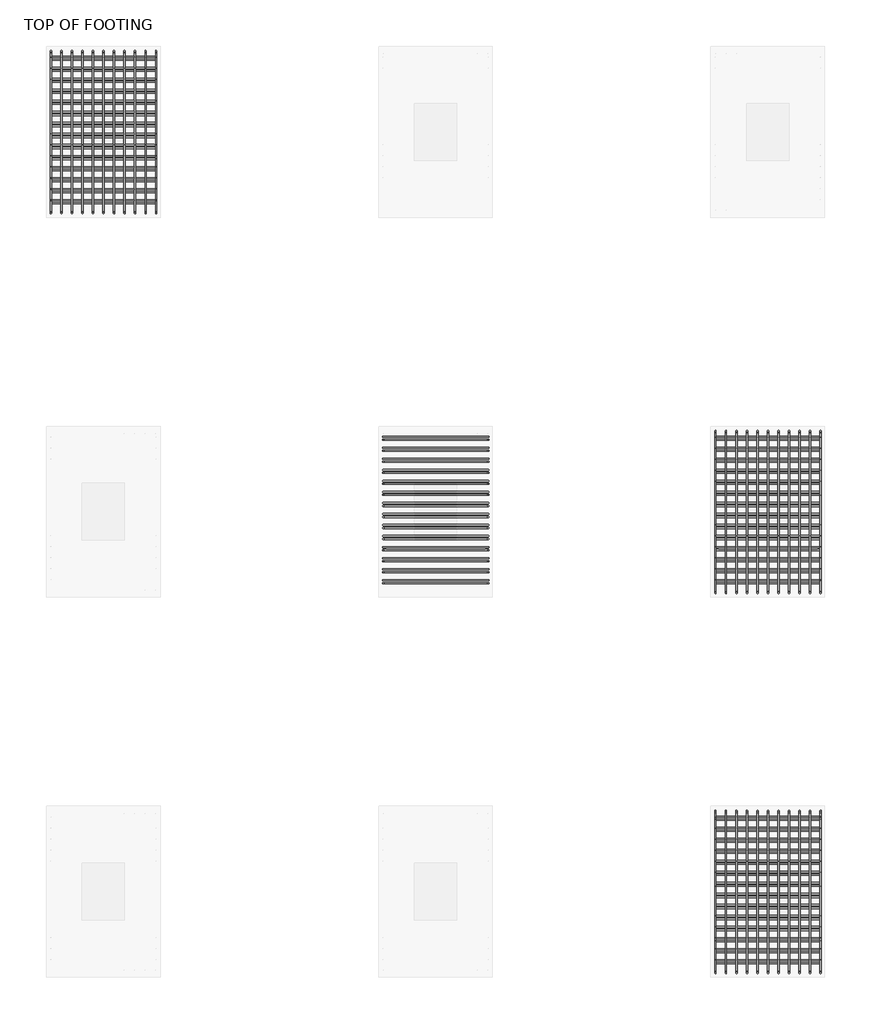
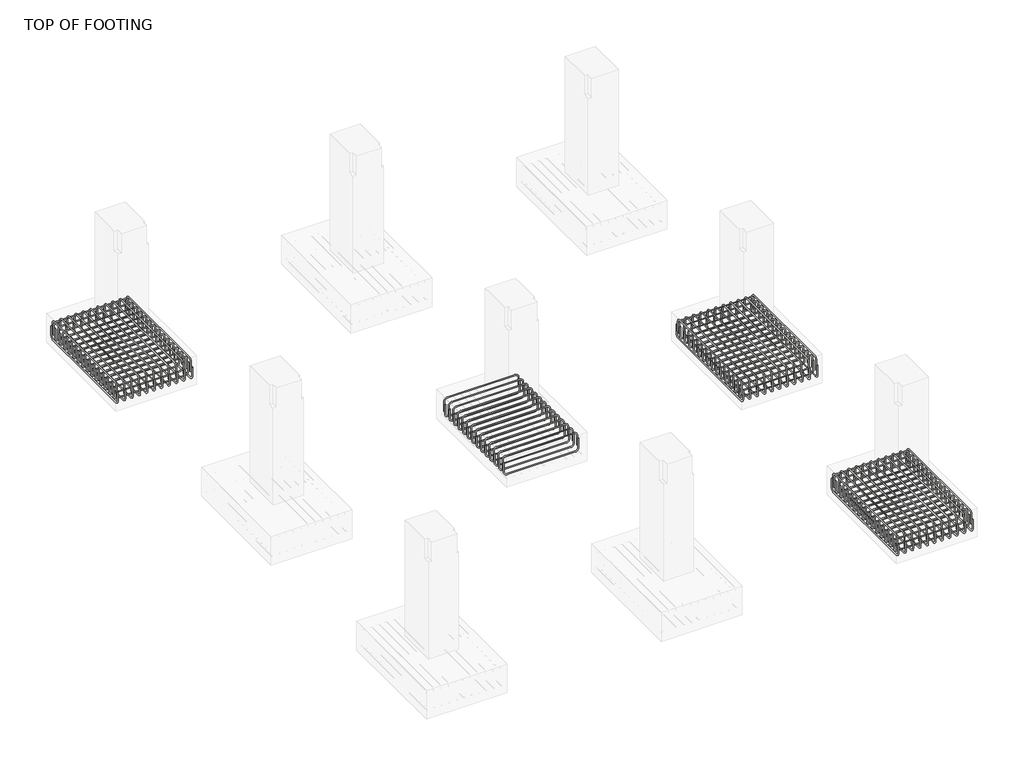
# One storey, part 10 of 11: 14 reinforcing bars.
"""IFC4 building model written with IfcOpenShell, lengths in millimetres."""

from ifc_helpers import new_model, si_unit, point, frame, origin, place, context, project, spatial, polyline, circle_curve, trimmed, segment, composite_curve, source, transform, mapped, element, save
from ifc_brep_helpers import swept_disk

model = new_model("IFC4")

# Units and contexts
model_context = context("Model", 3, world=origin())
ifc_project = project(units=[si_unit("LENGTHUNIT", "METRE", prefix="MILLI")], contexts=[model_context])

# Site, building, storey
site = spatial("IfcSite", under=ifc_project)
building = spatial("IfcBuilding", under=site)
storey = spatial("IfcBuildingStorey", under=building, Name="TOP OF FOOTING", Elevation=-1828.8)

# Reinforcing bars
placement = place(None, origin())
reinforcing_bar_shape = source(origin(), model_context, "Body", "SolidModel", [
    swept_disk(composite_curve([segment(polyline([(1683.7615906, 18549.4712443, -2012.1658531), (1683.7615906, 18549.4712443, -2159.4658531)]), True, "CONTINUOUS"), segment(trimmed(circle_curve(frame((1683.7615906, 18595.8212443, -2159.4658531), z_axis=(1.0, 0.0, 0.0), x_axis=(0.0, -46.35000000000218, 0.0)), 46.35), [point((1683.7615906, 18549.4712443, -2159.4658531))], [point((1683.7615906, 18595.8212443, -2205.8158531))], True, "CARTESIAN"), True, "CONTINUOUS"), segment(polyline([(1683.7615906, 18595.8212443, -2205.8158531), (1683.7615906, 20210.4212443, -2205.8158531)]), True, "CONTINUOUS"), segment(trimmed(circle_curve(frame((1683.7615906, 20210.4212443, -2159.4658531), z_axis=(1.0, 0.0, 0.0), x_axis=(0.0, 0.0, -46.34999999999991)), 46.35), [point((1683.7615906, 20210.4212443, -2205.8158531))], [point((1683.7615906, 20256.7712443, -2159.4658531))], True, "CARTESIAN"), True, "CONTINUOUS"), segment(polyline([(1683.7615906, 20256.7712443, -2159.4658531), (1683.7615906, 20256.7712443, -2012.1658531)]), True, "CONTINUOUS")], self_intersect=False), 6.35),
])
element("IfcReinforcingBar", 1, at=placement, inside=storey, context=model_context, shape_type="MappedRepresentation", body=[
    mapped(reinforcing_bar_shape, transform((0.0, 0.0, 0.0), x_axis=(1.0, 0.0, 0.0), y_axis=(0.0, 1.0, 0.0), z_axis=(0.0, 0.0, 1.0))),
    mapped(reinforcing_bar_shape, transform((-110.73, 0.0, 0.0), x_axis=(1.0, 0.0, 0.0), y_axis=(0.0, 1.0, 0.0), z_axis=(0.0, 0.0, 1.0))),
    mapped(reinforcing_bar_shape, transform((-221.46, 0.0, 0.0), x_axis=(1.0, 0.0, 0.0), y_axis=(0.0, 1.0, 0.0), z_axis=(0.0, 0.0, 1.0))),
    mapped(reinforcing_bar_shape, transform((-332.19, 0.0, 0.0), x_axis=(1.0, 0.0, 0.0), y_axis=(0.0, 1.0, 0.0), z_axis=(0.0, 0.0, 1.0))),
    mapped(reinforcing_bar_shape, transform((-442.92, 0.0, 0.0), x_axis=(1.0, 0.0, 0.0), y_axis=(0.0, 1.0, 0.0), z_axis=(0.0, 0.0, 1.0))),
    mapped(reinforcing_bar_shape, transform((-553.65, 0.0, 0.0), x_axis=(1.0, 0.0, 0.0), y_axis=(0.0, 1.0, 0.0), z_axis=(0.0, 0.0, 1.0))),
    mapped(reinforcing_bar_shape, transform((-664.38, 0.0, 0.0), x_axis=(1.0, 0.0, 0.0), y_axis=(0.0, 1.0, 0.0), z_axis=(0.0, 0.0, 1.0))),
    mapped(reinforcing_bar_shape, transform((-775.11, 0.0, 0.0), x_axis=(1.0, 0.0, 0.0), y_axis=(0.0, 1.0, 0.0), z_axis=(0.0, 0.0, 1.0))),
    mapped(reinforcing_bar_shape, transform((-885.84, 0.0, 0.0), x_axis=(1.0, 0.0, 0.0), y_axis=(0.0, 1.0, 0.0), z_axis=(0.0, 0.0, 1.0))),
    mapped(reinforcing_bar_shape, transform((-996.57, 0.0, 0.0), x_axis=(1.0, 0.0, 0.0), y_axis=(0.0, 1.0, 0.0), z_axis=(0.0, 0.0, 1.0))),
    mapped(reinforcing_bar_shape, transform((-1107.3, 0.0, 0.0), x_axis=(1.0, 0.0, 0.0), y_axis=(0.0, 1.0, 0.0), z_axis=(0.0, 0.0, 1.0))),
])
reinforcing_bar_2_shape = source(origin(), model_context, "Body", "SolidModel", [
    swept_disk(composite_curve([segment(polyline([(576.4615906, 18577.6603603, -2096.8914539), (576.4615906, 18577.6603603, -1949.5914539)]), True, "CONTINUOUS"), segment(trimmed(circle_curve(frame((576.4615906, 18624.0103603, -1949.5914539), z_axis=(-1.0, 0.0, 0.0), x_axis=(0.0, -46.349999999998545, 0.0)), 46.35), [point((576.4615906, 18577.6603603, -1949.5914539))], [point((576.4615906, 18624.0103603, -1903.2414539))], True, "CARTESIAN"), True, "CONTINUOUS"), segment(polyline([(576.4615906, 18624.0103603, -1903.2414539), (576.4615906, 20181.3238837, -1903.2414539)]), True, "CONTINUOUS"), segment(trimmed(circle_curve(frame((576.4615906, 20181.3238837, -1949.5914539), z_axis=(-1.0, 0.0, 0.0), x_axis=(0.0, 0.0, 46.350000000000136)), 46.35), [point((576.4615906, 20181.3238837, -1903.2414539))], [point((576.4615906, 20227.6738837, -1949.5914539))], True, "CARTESIAN"), True, "CONTINUOUS"), segment(polyline([(576.4615906, 20227.6738837, -1949.5914539), (576.4615906, 20227.6738837, -2096.8914539)]), True, "CONTINUOUS")], self_intersect=False), 6.35),
])
element("IfcReinforcingBar", 2, at=placement, inside=storey, context=model_context, shape_type="MappedRepresentation", body=[
    mapped(reinforcing_bar_2_shape, transform((0.0, 0.0, 0.0), x_axis=(1.0, 0.0, 0.0), y_axis=(0.0, 1.0, 0.0), z_axis=(0.0, 0.0, 1.0))),
    mapped(reinforcing_bar_2_shape, transform((110.73, 0.0, 0.0), x_axis=(1.0, 0.0, 0.0), y_axis=(0.0, 1.0, 0.0), z_axis=(0.0, 0.0, 1.0))),
    mapped(reinforcing_bar_2_shape, transform((221.46, 0.0, 0.0), x_axis=(1.0, 0.0, 0.0), y_axis=(0.0, 1.0, 0.0), z_axis=(0.0, 0.0, 1.0))),
    mapped(reinforcing_bar_2_shape, transform((332.19, 0.0, 0.0), x_axis=(1.0, 0.0, 0.0), y_axis=(0.0, 1.0, 0.0), z_axis=(0.0, 0.0, 1.0))),
    mapped(reinforcing_bar_2_shape, transform((442.92, 0.0, 0.0), x_axis=(1.0, 0.0, 0.0), y_axis=(0.0, 1.0, 0.0), z_axis=(0.0, 0.0, 1.0))),
    mapped(reinforcing_bar_2_shape, transform((553.65, 0.0, 0.0), x_axis=(1.0, 0.0, 0.0), y_axis=(0.0, 1.0, 0.0), z_axis=(0.0, 0.0, 1.0))),
    mapped(reinforcing_bar_2_shape, transform((664.38, 0.0, 0.0), x_axis=(1.0, 0.0, 0.0), y_axis=(0.0, 1.0, 0.0), z_axis=(0.0, 0.0, 1.0))),
    mapped(reinforcing_bar_2_shape, transform((775.11, 0.0, 0.0), x_axis=(1.0, 0.0, 0.0), y_axis=(0.0, 1.0, 0.0), z_axis=(0.0, 0.0, 1.0))),
    mapped(reinforcing_bar_2_shape, transform((885.84, 0.0, 0.0), x_axis=(1.0, 0.0, 0.0), y_axis=(0.0, 1.0, 0.0), z_axis=(0.0, 0.0, 1.0))),
    mapped(reinforcing_bar_2_shape, transform((996.57, 0.0, 0.0), x_axis=(1.0, 0.0, 0.0), y_axis=(0.0, 1.0, 0.0), z_axis=(0.0, 0.0, 1.0))),
    mapped(reinforcing_bar_2_shape, transform((1107.3, 0.0, 0.0), x_axis=(1.0, 0.0, 0.0), y_axis=(0.0, 1.0, 0.0), z_axis=(0.0, 0.0, 1.0))),
])
reinforcing_bar_3_shape = source(origin(), model_context, "Body", "SolidModel", [
    swept_disk(composite_curve([segment(polyline([(576.4615906, 18653.1930221, -1996.7664426), (576.4615906, 18653.1930221, -2144.0664426)]), True, "CONTINUOUS"), segment(trimmed(circle_curve(frame((622.8115906, 18653.1930221, -2144.0664426), z_axis=(0.0, -1.0, 0.0), x_axis=(-46.35000000000002, 0.0, 0.0)), 46.35), [point((576.4615906, 18653.1930221, -2144.0664426))], [point((622.8115906, 18653.1930221, -2190.4164426))], True, "CARTESIAN"), True, "CONTINUOUS"), segment(polyline([(622.8115906, 18653.1930221, -2190.4164426), (1637.4115906, 18653.1930221, -2190.4164426)]), True, "CONTINUOUS"), segment(trimmed(circle_curve(frame((1637.4115906, 18653.1930221, -2144.0664426), z_axis=(0.0, -1.0, 0.0), x_axis=(0.0, 0.0, -46.350000000000364)), 46.35), [point((1637.4115906, 18653.1930221, -2190.4164426))], [point((1683.7615906, 18653.1930221, -2144.0664426))], True, "CARTESIAN"), True, "CONTINUOUS"), segment(polyline([(1683.7615906, 18653.1930221, -2144.0664426), (1683.7615906, 18653.1930221, -1996.7664426)]), True, "CONTINUOUS")], self_intersect=False), 6.35),
])
element("IfcReinforcingBar", 3, at=placement, inside=storey, context=model_context, shape_type="MappedRepresentation", body=[
    mapped(reinforcing_bar_3_shape, transform((0.0, 0.0, 0.0), x_axis=(1.0, 0.0, 0.0), y_axis=(0.0, 1.0, 0.0), z_axis=(0.0, 0.0, 1.0))),
    mapped(reinforcing_bar_3_shape, transform((0.0, 116.2744005, 0.0), x_axis=(1.0, 0.0, 0.0), y_axis=(0.0, 1.0, 0.0), z_axis=(0.0, 0.0, 1.0))),
    mapped(reinforcing_bar_3_shape, transform((0.0, 232.5488009, 0.0), x_axis=(1.0, 0.0, 0.0), y_axis=(0.0, 1.0, 0.0), z_axis=(0.0, 0.0, 1.0))),
    mapped(reinforcing_bar_3_shape, transform((0.0, 348.8232014, 0.0), x_axis=(1.0, 0.0, 0.0), y_axis=(0.0, 1.0, 0.0), z_axis=(0.0, 0.0, 1.0))),
    mapped(reinforcing_bar_3_shape, transform((0.0, 465.0976018, 0.0), x_axis=(1.0, 0.0, 0.0), y_axis=(0.0, 1.0, 0.0), z_axis=(0.0, 0.0, 1.0))),
    mapped(reinforcing_bar_3_shape, transform((0.0, 581.3720023, 0.0), x_axis=(1.0, 0.0, 0.0), y_axis=(0.0, 1.0, 0.0), z_axis=(0.0, 0.0, 1.0))),
    mapped(reinforcing_bar_3_shape, transform((0.0, 697.6464027, 0.0), x_axis=(1.0, 0.0, 0.0), y_axis=(0.0, 1.0, 0.0), z_axis=(0.0, 0.0, 1.0))),
    mapped(reinforcing_bar_3_shape, transform((0.0, 813.9208032, 0.0), x_axis=(1.0, 0.0, 0.0), y_axis=(0.0, 1.0, 0.0), z_axis=(0.0, 0.0, 1.0))),
    mapped(reinforcing_bar_3_shape, transform((0.0, 930.1952036, 0.0), x_axis=(1.0, 0.0, 0.0), y_axis=(0.0, 1.0, 0.0), z_axis=(0.0, 0.0, 1.0))),
    mapped(reinforcing_bar_3_shape, transform((0.0, 1046.4696041, 0.0), x_axis=(1.0, 0.0, 0.0), y_axis=(0.0, 1.0, 0.0), z_axis=(0.0, 0.0, 1.0))),
    mapped(reinforcing_bar_3_shape, transform((0.0, 1162.7440045, 0.0), x_axis=(1.0, 0.0, 0.0), y_axis=(0.0, 1.0, 0.0), z_axis=(0.0, 0.0, 1.0))),
    mapped(reinforcing_bar_3_shape, transform((0.0, 1279.018405, 0.0), x_axis=(1.0, 0.0, 0.0), y_axis=(0.0, 1.0, 0.0), z_axis=(0.0, 0.0, 1.0))),
    mapped(reinforcing_bar_3_shape, transform((0.0, 1395.2928054, 0.0), x_axis=(1.0, 0.0, 0.0), y_axis=(0.0, 1.0, 0.0), z_axis=(0.0, 0.0, 1.0))),
    mapped(reinforcing_bar_3_shape, transform((0.0, 1511.5672059, 0.0), x_axis=(1.0, 0.0, 0.0), y_axis=(0.0, 1.0, 0.0), z_axis=(0.0, 0.0, 1.0))),
])
reinforcing_bar_4_shape = source(origin(), model_context, "Body", "SolidModel", [
    swept_disk(composite_curve([segment(polyline([(576.4615906, 20194.4257435, -2114.1958609), (576.4615906, 20194.4257435, -1966.8958609)]), True, "CONTINUOUS"), segment(trimmed(circle_curve(frame((622.8115906, 20194.4257435, -1966.8958609), z_axis=(0.0, 1.0, 0.0), x_axis=(-46.35000000000002, 0.0, 0.0)), 46.35), [point((576.4615906, 20194.4257435, -1966.8958609))], [point((622.8115906, 20194.4257435, -1920.5458609))], True, "CARTESIAN"), True, "CONTINUOUS"), segment(polyline([(622.8115906, 20194.4257435, -1920.5458609), (1637.4115906, 20194.4257435, -1920.5458609)]), True, "CONTINUOUS"), segment(trimmed(circle_curve(frame((1637.4115906, 20194.4257435, -1966.8958609), z_axis=(0.0, 1.0, 0.0), x_axis=(0.0, 0.0, 46.34999999999991)), 46.35), [point((1637.4115906, 20194.4257435, -1920.5458609))], [point((1683.7615906, 20194.4257435, -1966.8958609))], True, "CARTESIAN"), True, "CONTINUOUS"), segment(polyline([(1683.7615906, 20194.4257435, -1966.8958609), (1683.7615906, 20194.4257435, -2114.1958609)]), True, "CONTINUOUS")], self_intersect=False), 6.35),
])
element("IfcReinforcingBar", 4, at=placement, inside=storey, context=model_context, shape_type="MappedRepresentation", body=[
    mapped(reinforcing_bar_4_shape, transform((0.0, 0.0, 0.0), x_axis=(1.0, 0.0, 0.0), y_axis=(0.0, 1.0, 0.0), z_axis=(0.0, 0.0, 1.0))),
    mapped(reinforcing_bar_4_shape, transform((0.0, -116.1057918, 0.0), x_axis=(1.0, 0.0, 0.0), y_axis=(0.0, 1.0, 0.0), z_axis=(0.0, 0.0, 1.0))),
    mapped(reinforcing_bar_4_shape, transform((0.0, -232.2115836, 0.0), x_axis=(1.0, 0.0, 0.0), y_axis=(0.0, 1.0, 0.0), z_axis=(0.0, 0.0, 1.0))),
    mapped(reinforcing_bar_4_shape, transform((0.0, -348.3173754, 0.0), x_axis=(1.0, 0.0, 0.0), y_axis=(0.0, 1.0, 0.0), z_axis=(0.0, 0.0, 1.0))),
    mapped(reinforcing_bar_4_shape, transform((0.0, -464.4231672, 0.0), x_axis=(1.0, 0.0, 0.0), y_axis=(0.0, 1.0, 0.0), z_axis=(0.0, 0.0, 1.0))),
    mapped(reinforcing_bar_4_shape, transform((0.0, -580.528959, 0.0), x_axis=(1.0, 0.0, 0.0), y_axis=(0.0, 1.0, 0.0), z_axis=(0.0, 0.0, 1.0))),
    mapped(reinforcing_bar_4_shape, transform((0.0, -696.6347508, 0.0), x_axis=(1.0, 0.0, 0.0), y_axis=(0.0, 1.0, 0.0), z_axis=(0.0, 0.0, 1.0))),
    mapped(reinforcing_bar_4_shape, transform((0.0, -812.7405426, 0.0), x_axis=(1.0, 0.0, 0.0), y_axis=(0.0, 1.0, 0.0), z_axis=(0.0, 0.0, 1.0))),
    mapped(reinforcing_bar_4_shape, transform((0.0, -928.8463344, 0.0), x_axis=(1.0, 0.0, 0.0), y_axis=(0.0, 1.0, 0.0), z_axis=(0.0, 0.0, 1.0))),
    mapped(reinforcing_bar_4_shape, transform((0.0, -1044.9521262, 0.0), x_axis=(1.0, 0.0, 0.0), y_axis=(0.0, 1.0, 0.0), z_axis=(0.0, 0.0, 1.0))),
    mapped(reinforcing_bar_4_shape, transform((0.0, -1161.057918, 0.0), x_axis=(1.0, 0.0, 0.0), y_axis=(0.0, 1.0, 0.0), z_axis=(0.0, 0.0, 1.0))),
    mapped(reinforcing_bar_4_shape, transform((0.0, -1277.1637098, 0.0), x_axis=(1.0, 0.0, 0.0), y_axis=(0.0, 1.0, 0.0), z_axis=(0.0, 0.0, 1.0))),
    mapped(reinforcing_bar_4_shape, transform((0.0, -1393.2695016, 0.0), x_axis=(1.0, 0.0, 0.0), y_axis=(0.0, 1.0, 0.0), z_axis=(0.0, 0.0, 1.0))),
    mapped(reinforcing_bar_4_shape, transform((0.0, -1509.3752934, 0.0), x_axis=(1.0, 0.0, 0.0), y_axis=(0.0, 1.0, 0.0), z_axis=(0.0, 0.0, 1.0))),
])
reinforcing_bar_5_shape = source(origin(), model_context, "Body", "SolidModel", [
    swept_disk(composite_curve([segment(polyline([(8683.7615906, 10549.4712443, -2012.1658531), (8683.7615906, 10549.4712443, -2159.4658531)]), True, "CONTINUOUS"), segment(trimmed(circle_curve(frame((8683.7615906, 10595.8212443, -2159.4658531), z_axis=(1.0, 0.0, 0.0), x_axis=(0.0, -46.349999999998545, 0.0)), 46.35), [point((8683.7615906, 10549.4712443, -2159.4658531))], [point((8683.7615906, 10595.8212443, -2205.8158531))], True, "CARTESIAN"), True, "CONTINUOUS"), segment(polyline([(8683.7615906, 10595.8212443, -2205.8158531), (8683.7615906, 12210.4212443, -2205.8158531)]), True, "CONTINUOUS"), segment(trimmed(circle_curve(frame((8683.7615906, 12210.4212443, -2159.4658531), z_axis=(1.0, 0.0, 0.0), x_axis=(0.0, 0.0, -46.34999999999991)), 46.35), [point((8683.7615906, 12210.4212443, -2205.8158531))], [point((8683.7615906, 12256.7712443, -2159.4658531))], True, "CARTESIAN"), True, "CONTINUOUS"), segment(polyline([(8683.7615906, 12256.7712443, -2159.4658531), (8683.7615906, 12256.7712443, -2012.1658531)]), True, "CONTINUOUS")], self_intersect=False), 6.35),
])
element("IfcReinforcingBar", 5, at=placement, inside=storey, context=model_context, shape_type="MappedRepresentation", body=[
    mapped(reinforcing_bar_5_shape, transform((0.0, 0.0, 0.0), x_axis=(1.0, 0.0, 0.0), y_axis=(0.0, 1.0, 0.0), z_axis=(0.0, 0.0, 1.0))),
    mapped(reinforcing_bar_5_shape, transform((-110.73, 0.0, 0.0), x_axis=(1.0, 0.0, 0.0), y_axis=(0.0, 1.0, 0.0), z_axis=(0.0, 0.0, 1.0))),
    mapped(reinforcing_bar_5_shape, transform((-221.46, 0.0, 0.0), x_axis=(1.0, 0.0, 0.0), y_axis=(0.0, 1.0, 0.0), z_axis=(0.0, 0.0, 1.0))),
    mapped(reinforcing_bar_5_shape, transform((-332.19, 0.0, 0.0), x_axis=(1.0, 0.0, 0.0), y_axis=(0.0, 1.0, 0.0), z_axis=(0.0, 0.0, 1.0))),
    mapped(reinforcing_bar_5_shape, transform((-442.92, 0.0, 0.0), x_axis=(1.0, 0.0, 0.0), y_axis=(0.0, 1.0, 0.0), z_axis=(0.0, 0.0, 1.0))),
    mapped(reinforcing_bar_5_shape, transform((-553.65, 0.0, 0.0), x_axis=(1.0, 0.0, 0.0), y_axis=(0.0, 1.0, 0.0), z_axis=(0.0, 0.0, 1.0))),
    mapped(reinforcing_bar_5_shape, transform((-664.38, 0.0, 0.0), x_axis=(1.0, 0.0, 0.0), y_axis=(0.0, 1.0, 0.0), z_axis=(0.0, 0.0, 1.0))),
    mapped(reinforcing_bar_5_shape, transform((-775.11, 0.0, 0.0), x_axis=(1.0, 0.0, 0.0), y_axis=(0.0, 1.0, 0.0), z_axis=(0.0, 0.0, 1.0))),
    mapped(reinforcing_bar_5_shape, transform((-885.84, 0.0, 0.0), x_axis=(1.0, 0.0, 0.0), y_axis=(0.0, 1.0, 0.0), z_axis=(0.0, 0.0, 1.0))),
    mapped(reinforcing_bar_5_shape, transform((-996.57, 0.0, 0.0), x_axis=(1.0, 0.0, 0.0), y_axis=(0.0, 1.0, 0.0), z_axis=(0.0, 0.0, 1.0))),
    mapped(reinforcing_bar_5_shape, transform((-1107.3, 0.0, 0.0), x_axis=(1.0, 0.0, 0.0), y_axis=(0.0, 1.0, 0.0), z_axis=(0.0, 0.0, 1.0))),
])
reinforcing_bar_6_shape = source(origin(), model_context, "Body", "SolidModel", [
    swept_disk(composite_curve([segment(polyline([(7576.4615906, 10577.6603603, -2096.8914539), (7576.4615906, 10577.6603603, -1949.5914539)]), True, "CONTINUOUS"), segment(trimmed(circle_curve(frame((7576.4615906, 10624.0103603, -1949.5914539), z_axis=(-1.0, 0.0, 0.0), x_axis=(0.0, -46.350000000000364, 0.0)), 46.35), [point((7576.4615906, 10577.6603603, -1949.5914539))], [point((7576.4615906, 10624.0103603, -1903.2414539))], True, "CARTESIAN"), True, "CONTINUOUS"), segment(polyline([(7576.4615906, 10624.0103603, -1903.2414539), (7576.4615906, 12181.3238837, -1903.2414539)]), True, "CONTINUOUS"), segment(trimmed(circle_curve(frame((7576.4615906, 12181.3238837, -1949.5914539), z_axis=(-1.0, 0.0, 0.0), x_axis=(0.0, 0.0, 46.350000000000136)), 46.35), [point((7576.4615906, 12181.3238837, -1903.2414539))], [point((7576.4615906, 12227.6738837, -1949.5914539))], True, "CARTESIAN"), True, "CONTINUOUS"), segment(polyline([(7576.4615906, 12227.6738837, -1949.5914539), (7576.4615906, 12227.6738837, -2096.8914539)]), True, "CONTINUOUS")], self_intersect=False), 6.35),
])
element("IfcReinforcingBar", 6, at=placement, inside=storey, context=model_context, shape_type="MappedRepresentation", body=[
    mapped(reinforcing_bar_6_shape, transform((0.0, 0.0, 0.0), x_axis=(1.0, 0.0, 0.0), y_axis=(0.0, 1.0, 0.0), z_axis=(0.0, 0.0, 1.0))),
    mapped(reinforcing_bar_6_shape, transform((110.73, 0.0, 0.0), x_axis=(1.0, 0.0, 0.0), y_axis=(0.0, 1.0, 0.0), z_axis=(0.0, 0.0, 1.0))),
    mapped(reinforcing_bar_6_shape, transform((221.46, 0.0, 0.0), x_axis=(1.0, 0.0, 0.0), y_axis=(0.0, 1.0, 0.0), z_axis=(0.0, 0.0, 1.0))),
    mapped(reinforcing_bar_6_shape, transform((332.19, 0.0, 0.0), x_axis=(1.0, 0.0, 0.0), y_axis=(0.0, 1.0, 0.0), z_axis=(0.0, 0.0, 1.0))),
    mapped(reinforcing_bar_6_shape, transform((442.92, 0.0, 0.0), x_axis=(1.0, 0.0, 0.0), y_axis=(0.0, 1.0, 0.0), z_axis=(0.0, 0.0, 1.0))),
    mapped(reinforcing_bar_6_shape, transform((553.65, 0.0, 0.0), x_axis=(1.0, 0.0, 0.0), y_axis=(0.0, 1.0, 0.0), z_axis=(0.0, 0.0, 1.0))),
    mapped(reinforcing_bar_6_shape, transform((664.38, 0.0, 0.0), x_axis=(1.0, 0.0, 0.0), y_axis=(0.0, 1.0, 0.0), z_axis=(0.0, 0.0, 1.0))),
    mapped(reinforcing_bar_6_shape, transform((775.11, 0.0, 0.0), x_axis=(1.0, 0.0, 0.0), y_axis=(0.0, 1.0, 0.0), z_axis=(0.0, 0.0, 1.0))),
    mapped(reinforcing_bar_6_shape, transform((885.84, 0.0, 0.0), x_axis=(1.0, 0.0, 0.0), y_axis=(0.0, 1.0, 0.0), z_axis=(0.0, 0.0, 1.0))),
    mapped(reinforcing_bar_6_shape, transform((996.57, 0.0, 0.0), x_axis=(1.0, 0.0, 0.0), y_axis=(0.0, 1.0, 0.0), z_axis=(0.0, 0.0, 1.0))),
    mapped(reinforcing_bar_6_shape, transform((1107.3, 0.0, 0.0), x_axis=(1.0, 0.0, 0.0), y_axis=(0.0, 1.0, 0.0), z_axis=(0.0, 0.0, 1.0))),
])
reinforcing_bar_7_shape = source(origin(), model_context, "Body", "SolidModel", [
    swept_disk(composite_curve([segment(polyline([(7576.4615906, 10653.1930221, -1996.7664426), (7576.4615906, 10653.1930221, -2144.0664426)]), True, "CONTINUOUS"), segment(trimmed(circle_curve(frame((7622.8115906, 10653.1930221, -2144.0664426), z_axis=(0.0, -1.0, 0.0), x_axis=(-46.350000000000364, 0.0, 0.0)), 46.35), [point((7576.4615906, 10653.1930221, -2144.0664426))], [point((7622.8115906, 10653.1930221, -2190.4164426))], True, "CARTESIAN"), True, "CONTINUOUS"), segment(polyline([(7622.8115906, 10653.1930221, -2190.4164426), (8637.4115906, 10653.1930221, -2190.4164426)]), True, "CONTINUOUS"), segment(trimmed(circle_curve(frame((8637.4115906, 10653.1930221, -2144.0664426), z_axis=(0.0, -1.0, 0.0), x_axis=(0.0, 0.0, -46.350000000000364)), 46.35), [point((8637.4115906, 10653.1930221, -2190.4164426))], [point((8683.7615906, 10653.1930221, -2144.0664426))], True, "CARTESIAN"), True, "CONTINUOUS"), segment(polyline([(8683.7615906, 10653.1930221, -2144.0664426), (8683.7615906, 10653.1930221, -1996.7664426)]), True, "CONTINUOUS")], self_intersect=False), 6.35),
])
element("IfcReinforcingBar", 7, at=placement, inside=storey, context=model_context, shape_type="MappedRepresentation", body=[
    mapped(reinforcing_bar_7_shape, transform((0.0, 0.0, 0.0), x_axis=(1.0, 0.0, 0.0), y_axis=(0.0, 1.0, 0.0), z_axis=(0.0, 0.0, 1.0))),
    mapped(reinforcing_bar_7_shape, transform((0.0, 116.2744005, 0.0), x_axis=(1.0, 0.0, 0.0), y_axis=(0.0, 1.0, 0.0), z_axis=(0.0, 0.0, 1.0))),
    mapped(reinforcing_bar_7_shape, transform((0.0, 232.5488009, 0.0), x_axis=(1.0, 0.0, 0.0), y_axis=(0.0, 1.0, 0.0), z_axis=(0.0, 0.0, 1.0))),
    mapped(reinforcing_bar_7_shape, transform((0.0, 348.8232014, 0.0), x_axis=(1.0, 0.0, 0.0), y_axis=(0.0, 1.0, 0.0), z_axis=(0.0, 0.0, 1.0))),
    mapped(reinforcing_bar_7_shape, transform((0.0, 465.0976018, 0.0), x_axis=(1.0, 0.0, 0.0), y_axis=(0.0, 1.0, 0.0), z_axis=(0.0, 0.0, 1.0))),
    mapped(reinforcing_bar_7_shape, transform((0.0, 581.3720023, 0.0), x_axis=(1.0, 0.0, 0.0), y_axis=(0.0, 1.0, 0.0), z_axis=(0.0, 0.0, 1.0))),
    mapped(reinforcing_bar_7_shape, transform((0.0, 697.6464027, 0.0), x_axis=(1.0, 0.0, 0.0), y_axis=(0.0, 1.0, 0.0), z_axis=(0.0, 0.0, 1.0))),
    mapped(reinforcing_bar_7_shape, transform((0.0, 813.9208032, 0.0), x_axis=(1.0, 0.0, 0.0), y_axis=(0.0, 1.0, 0.0), z_axis=(0.0, 0.0, 1.0))),
    mapped(reinforcing_bar_7_shape, transform((0.0, 930.1952036, 0.0), x_axis=(1.0, 0.0, 0.0), y_axis=(0.0, 1.0, 0.0), z_axis=(0.0, 0.0, 1.0))),
    mapped(reinforcing_bar_7_shape, transform((0.0, 1046.4696041, 0.0), x_axis=(1.0, 0.0, 0.0), y_axis=(0.0, 1.0, 0.0), z_axis=(0.0, 0.0, 1.0))),
    mapped(reinforcing_bar_7_shape, transform((0.0, 1162.7440045, 0.0), x_axis=(1.0, 0.0, 0.0), y_axis=(0.0, 1.0, 0.0), z_axis=(0.0, 0.0, 1.0))),
    mapped(reinforcing_bar_7_shape, transform((0.0, 1279.018405, 0.0), x_axis=(1.0, 0.0, 0.0), y_axis=(0.0, 1.0, 0.0), z_axis=(0.0, 0.0, 1.0))),
    mapped(reinforcing_bar_7_shape, transform((0.0, 1395.2928054, 0.0), x_axis=(1.0, 0.0, 0.0), y_axis=(0.0, 1.0, 0.0), z_axis=(0.0, 0.0, 1.0))),
    mapped(reinforcing_bar_7_shape, transform((0.0, 1511.5672059, 0.0), x_axis=(1.0, 0.0, 0.0), y_axis=(0.0, 1.0, 0.0), z_axis=(0.0, 0.0, 1.0))),
])
reinforcing_bar_8_shape = source(origin(), model_context, "Body", "SolidModel", [
    swept_disk(composite_curve([segment(polyline([(7576.4615906, 12194.4257435, -2114.1958609), (7576.4615906, 12194.4257435, -1966.8958609)]), True, "CONTINUOUS"), segment(trimmed(circle_curve(frame((7622.8115906, 12194.4257435, -1966.8958609), z_axis=(0.0, 1.0, 0.0), x_axis=(-46.350000000000364, 0.0, 0.0)), 46.35), [point((7576.4615906, 12194.4257435, -1966.8958609))], [point((7622.8115906, 12194.4257435, -1920.5458609))], True, "CARTESIAN"), True, "CONTINUOUS"), segment(polyline([(7622.8115906, 12194.4257435, -1920.5458609), (8637.4115906, 12194.4257435, -1920.5458609)]), True, "CONTINUOUS"), segment(trimmed(circle_curve(frame((8637.4115906, 12194.4257435, -1966.8958609), z_axis=(0.0, 1.0, 0.0), x_axis=(0.0, 0.0, 46.34999999999991)), 46.35), [point((8637.4115906, 12194.4257435, -1920.5458609))], [point((8683.7615906, 12194.4257435, -1966.8958609))], True, "CARTESIAN"), True, "CONTINUOUS"), segment(polyline([(8683.7615906, 12194.4257435, -1966.8958609), (8683.7615906, 12194.4257435, -2114.1958609)]), True, "CONTINUOUS")], self_intersect=False), 6.35),
])
element("IfcReinforcingBar", 8, at=placement, inside=storey, context=model_context, shape_type="MappedRepresentation", body=[
    mapped(reinforcing_bar_8_shape, transform((0.0, 0.0, 0.0), x_axis=(1.0, 0.0, 0.0), y_axis=(0.0, 1.0, 0.0), z_axis=(0.0, 0.0, 1.0))),
    mapped(reinforcing_bar_8_shape, transform((0.0, -116.1057918, 0.0), x_axis=(1.0, 0.0, 0.0), y_axis=(0.0, 1.0, 0.0), z_axis=(0.0, 0.0, 1.0))),
    mapped(reinforcing_bar_8_shape, transform((0.0, -232.2115836, 0.0), x_axis=(1.0, 0.0, 0.0), y_axis=(0.0, 1.0, 0.0), z_axis=(0.0, 0.0, 1.0))),
    mapped(reinforcing_bar_8_shape, transform((0.0, -348.3173754, 0.0), x_axis=(1.0, 0.0, 0.0), y_axis=(0.0, 1.0, 0.0), z_axis=(0.0, 0.0, 1.0))),
    mapped(reinforcing_bar_8_shape, transform((0.0, -464.4231672, 0.0), x_axis=(1.0, 0.0, 0.0), y_axis=(0.0, 1.0, 0.0), z_axis=(0.0, 0.0, 1.0))),
    mapped(reinforcing_bar_8_shape, transform((0.0, -580.528959, 0.0), x_axis=(1.0, 0.0, 0.0), y_axis=(0.0, 1.0, 0.0), z_axis=(0.0, 0.0, 1.0))),
    mapped(reinforcing_bar_8_shape, transform((0.0, -696.6347508, 0.0), x_axis=(1.0, 0.0, 0.0), y_axis=(0.0, 1.0, 0.0), z_axis=(0.0, 0.0, 1.0))),
    mapped(reinforcing_bar_8_shape, transform((0.0, -812.7405426, 0.0), x_axis=(1.0, 0.0, 0.0), y_axis=(0.0, 1.0, 0.0), z_axis=(0.0, 0.0, 1.0))),
    mapped(reinforcing_bar_8_shape, transform((0.0, -928.8463344, 0.0), x_axis=(1.0, 0.0, 0.0), y_axis=(0.0, 1.0, 0.0), z_axis=(0.0, 0.0, 1.0))),
    mapped(reinforcing_bar_8_shape, transform((0.0, -1044.9521262, 0.0), x_axis=(1.0, 0.0, 0.0), y_axis=(0.0, 1.0, 0.0), z_axis=(0.0, 0.0, 1.0))),
    mapped(reinforcing_bar_8_shape, transform((0.0, -1161.057918, 0.0), x_axis=(1.0, 0.0, 0.0), y_axis=(0.0, 1.0, 0.0), z_axis=(0.0, 0.0, 1.0))),
    mapped(reinforcing_bar_8_shape, transform((0.0, -1277.1637098, 0.0), x_axis=(1.0, 0.0, 0.0), y_axis=(0.0, 1.0, 0.0), z_axis=(0.0, 0.0, 1.0))),
    mapped(reinforcing_bar_8_shape, transform((0.0, -1393.2695016, 0.0), x_axis=(1.0, 0.0, 0.0), y_axis=(0.0, 1.0, 0.0), z_axis=(0.0, 0.0, 1.0))),
    mapped(reinforcing_bar_8_shape, transform((0.0, -1509.3752934, 0.0), x_axis=(1.0, 0.0, 0.0), y_axis=(0.0, 1.0, 0.0), z_axis=(0.0, 0.0, 1.0))),
])
reinforcing_bar_9_shape = source(origin(), model_context, "Body", "SolidModel", [
    swept_disk(composite_curve([segment(polyline([(8683.7615906, 14549.4712443, -2012.1658531), (8683.7615906, 14549.4712443, -2159.4658531)]), True, "CONTINUOUS"), segment(trimmed(circle_curve(frame((8683.7615906, 14595.8212443, -2159.4658531), z_axis=(1.0, 0.0, 0.0), x_axis=(0.0, -46.349999999998545, 0.0)), 46.35), [point((8683.7615906, 14549.4712443, -2159.4658531))], [point((8683.7615906, 14595.8212443, -2205.8158531))], True, "CARTESIAN"), True, "CONTINUOUS"), segment(polyline([(8683.7615906, 14595.8212443, -2205.8158531), (8683.7615906, 16210.4212443, -2205.8158531)]), True, "CONTINUOUS"), segment(trimmed(circle_curve(frame((8683.7615906, 16210.4212443, -2159.4658531), z_axis=(1.0, 0.0, 0.0), x_axis=(0.0, 0.0, -46.34999999999991)), 46.35), [point((8683.7615906, 16210.4212443, -2205.8158531))], [point((8683.7615906, 16256.7712443, -2159.4658531))], True, "CARTESIAN"), True, "CONTINUOUS"), segment(polyline([(8683.7615906, 16256.7712443, -2159.4658531), (8683.7615906, 16256.7712443, -2012.1658531)]), True, "CONTINUOUS")], self_intersect=False), 6.35),
])
element("IfcReinforcingBar", 9, at=placement, inside=storey, context=model_context, shape_type="MappedRepresentation", body=[
    mapped(reinforcing_bar_9_shape, transform((0.0, 0.0, 0.0), x_axis=(1.0, 0.0, 0.0), y_axis=(0.0, 1.0, 0.0), z_axis=(0.0, 0.0, 1.0))),
    mapped(reinforcing_bar_9_shape, transform((-110.73, 0.0, 0.0), x_axis=(1.0, 0.0, 0.0), y_axis=(0.0, 1.0, 0.0), z_axis=(0.0, 0.0, 1.0))),
    mapped(reinforcing_bar_9_shape, transform((-221.46, 0.0, 0.0), x_axis=(1.0, 0.0, 0.0), y_axis=(0.0, 1.0, 0.0), z_axis=(0.0, 0.0, 1.0))),
    mapped(reinforcing_bar_9_shape, transform((-332.19, 0.0, 0.0), x_axis=(1.0, 0.0, 0.0), y_axis=(0.0, 1.0, 0.0), z_axis=(0.0, 0.0, 1.0))),
    mapped(reinforcing_bar_9_shape, transform((-442.92, 0.0, 0.0), x_axis=(1.0, 0.0, 0.0), y_axis=(0.0, 1.0, 0.0), z_axis=(0.0, 0.0, 1.0))),
    mapped(reinforcing_bar_9_shape, transform((-553.65, 0.0, 0.0), x_axis=(1.0, 0.0, 0.0), y_axis=(0.0, 1.0, 0.0), z_axis=(0.0, 0.0, 1.0))),
    mapped(reinforcing_bar_9_shape, transform((-664.38, 0.0, 0.0), x_axis=(1.0, 0.0, 0.0), y_axis=(0.0, 1.0, 0.0), z_axis=(0.0, 0.0, 1.0))),
    mapped(reinforcing_bar_9_shape, transform((-775.11, 0.0, 0.0), x_axis=(1.0, 0.0, 0.0), y_axis=(0.0, 1.0, 0.0), z_axis=(0.0, 0.0, 1.0))),
    mapped(reinforcing_bar_9_shape, transform((-885.84, 0.0, 0.0), x_axis=(1.0, 0.0, 0.0), y_axis=(0.0, 1.0, 0.0), z_axis=(0.0, 0.0, 1.0))),
    mapped(reinforcing_bar_9_shape, transform((-996.57, 0.0, 0.0), x_axis=(1.0, 0.0, 0.0), y_axis=(0.0, 1.0, 0.0), z_axis=(0.0, 0.0, 1.0))),
    mapped(reinforcing_bar_9_shape, transform((-1107.3, 0.0, 0.0), x_axis=(1.0, 0.0, 0.0), y_axis=(0.0, 1.0, 0.0), z_axis=(0.0, 0.0, 1.0))),
])
reinforcing_bar_10_shape = source(origin(), model_context, "Body", "SolidModel", [
    swept_disk(composite_curve([segment(polyline([(7576.4615906, 14577.6603603, -2096.8914539), (7576.4615906, 14577.6603603, -1949.5914539)]), True, "CONTINUOUS"), segment(trimmed(circle_curve(frame((7576.4615906, 14624.0103603, -1949.5914539), z_axis=(-1.0, 0.0, 0.0), x_axis=(0.0, -46.350000000000364, 0.0)), 46.35), [point((7576.4615906, 14577.6603603, -1949.5914539))], [point((7576.4615906, 14624.0103603, -1903.2414539))], True, "CARTESIAN"), True, "CONTINUOUS"), segment(polyline([(7576.4615906, 14624.0103603, -1903.2414539), (7576.4615906, 16181.3238837, -1903.2414539)]), True, "CONTINUOUS"), segment(trimmed(circle_curve(frame((7576.4615906, 16181.3238837, -1949.5914539), z_axis=(-1.0, 0.0, 0.0), x_axis=(0.0, 0.0, 46.350000000000136)), 46.35), [point((7576.4615906, 16181.3238837, -1903.2414539))], [point((7576.4615906, 16227.6738837, -1949.5914539))], True, "CARTESIAN"), True, "CONTINUOUS"), segment(polyline([(7576.4615906, 16227.6738837, -1949.5914539), (7576.4615906, 16227.6738837, -2096.8914539)]), True, "CONTINUOUS")], self_intersect=False), 6.35),
])
element("IfcReinforcingBar", 10, at=placement, inside=storey, context=model_context, shape_type="MappedRepresentation", body=[
    mapped(reinforcing_bar_10_shape, transform((0.0, 0.0, 0.0), x_axis=(1.0, 0.0, 0.0), y_axis=(0.0, 1.0, 0.0), z_axis=(0.0, 0.0, 1.0))),
    mapped(reinforcing_bar_10_shape, transform((110.73, 0.0, 0.0), x_axis=(1.0, 0.0, 0.0), y_axis=(0.0, 1.0, 0.0), z_axis=(0.0, 0.0, 1.0))),
    mapped(reinforcing_bar_10_shape, transform((221.46, 0.0, 0.0), x_axis=(1.0, 0.0, 0.0), y_axis=(0.0, 1.0, 0.0), z_axis=(0.0, 0.0, 1.0))),
    mapped(reinforcing_bar_10_shape, transform((332.19, 0.0, 0.0), x_axis=(1.0, 0.0, 0.0), y_axis=(0.0, 1.0, 0.0), z_axis=(0.0, 0.0, 1.0))),
    mapped(reinforcing_bar_10_shape, transform((442.92, 0.0, 0.0), x_axis=(1.0, 0.0, 0.0), y_axis=(0.0, 1.0, 0.0), z_axis=(0.0, 0.0, 1.0))),
    mapped(reinforcing_bar_10_shape, transform((553.65, 0.0, 0.0), x_axis=(1.0, 0.0, 0.0), y_axis=(0.0, 1.0, 0.0), z_axis=(0.0, 0.0, 1.0))),
    mapped(reinforcing_bar_10_shape, transform((664.38, 0.0, 0.0), x_axis=(1.0, 0.0, 0.0), y_axis=(0.0, 1.0, 0.0), z_axis=(0.0, 0.0, 1.0))),
    mapped(reinforcing_bar_10_shape, transform((775.11, 0.0, 0.0), x_axis=(1.0, 0.0, 0.0), y_axis=(0.0, 1.0, 0.0), z_axis=(0.0, 0.0, 1.0))),
    mapped(reinforcing_bar_10_shape, transform((885.84, 0.0, 0.0), x_axis=(1.0, 0.0, 0.0), y_axis=(0.0, 1.0, 0.0), z_axis=(0.0, 0.0, 1.0))),
    mapped(reinforcing_bar_10_shape, transform((996.57, 0.0, 0.0), x_axis=(1.0, 0.0, 0.0), y_axis=(0.0, 1.0, 0.0), z_axis=(0.0, 0.0, 1.0))),
    mapped(reinforcing_bar_10_shape, transform((1107.3, 0.0, 0.0), x_axis=(1.0, 0.0, 0.0), y_axis=(0.0, 1.0, 0.0), z_axis=(0.0, 0.0, 1.0))),
])
reinforcing_bar_11_shape = source(origin(), model_context, "Body", "SolidModel", [
    swept_disk(composite_curve([segment(polyline([(7576.4615906, 14653.1930221, -1996.7664426), (7576.4615906, 14653.1930221, -2144.0664426)]), True, "CONTINUOUS"), segment(trimmed(circle_curve(frame((7622.8115906, 14653.1930221, -2144.0664426), z_axis=(0.0, -1.0, 0.0), x_axis=(-46.350000000000364, 0.0, 0.0)), 46.35), [point((7576.4615906, 14653.1930221, -2144.0664426))], [point((7622.8115906, 14653.1930221, -2190.4164426))], True, "CARTESIAN"), True, "CONTINUOUS"), segment(polyline([(7622.8115906, 14653.1930221, -2190.4164426), (8637.4115906, 14653.1930221, -2190.4164426)]), True, "CONTINUOUS"), segment(trimmed(circle_curve(frame((8637.4115906, 14653.1930221, -2144.0664426), z_axis=(0.0, -1.0, 0.0), x_axis=(0.0, 0.0, -46.350000000000364)), 46.35), [point((8637.4115906, 14653.1930221, -2190.4164426))], [point((8683.7615906, 14653.1930221, -2144.0664426))], True, "CARTESIAN"), True, "CONTINUOUS"), segment(polyline([(8683.7615906, 14653.1930221, -2144.0664426), (8683.7615906, 14653.1930221, -1996.7664426)]), True, "CONTINUOUS")], self_intersect=False), 6.35),
])
element("IfcReinforcingBar", 11, at=placement, inside=storey, context=model_context, shape_type="MappedRepresentation", body=[
    mapped(reinforcing_bar_11_shape, transform((0.0, 0.0, 0.0), x_axis=(1.0, 0.0, 0.0), y_axis=(0.0, 1.0, 0.0), z_axis=(0.0, 0.0, 1.0))),
    mapped(reinforcing_bar_11_shape, transform((0.0, 116.2744005, 0.0), x_axis=(1.0, 0.0, 0.0), y_axis=(0.0, 1.0, 0.0), z_axis=(0.0, 0.0, 1.0))),
    mapped(reinforcing_bar_11_shape, transform((0.0, 232.5488009, 0.0), x_axis=(1.0, 0.0, 0.0), y_axis=(0.0, 1.0, 0.0), z_axis=(0.0, 0.0, 1.0))),
    mapped(reinforcing_bar_11_shape, transform((0.0, 348.8232014, 0.0), x_axis=(1.0, 0.0, 0.0), y_axis=(0.0, 1.0, 0.0), z_axis=(0.0, 0.0, 1.0))),
    mapped(reinforcing_bar_11_shape, transform((0.0, 465.0976018, 0.0), x_axis=(1.0, 0.0, 0.0), y_axis=(0.0, 1.0, 0.0), z_axis=(0.0, 0.0, 1.0))),
    mapped(reinforcing_bar_11_shape, transform((0.0, 581.3720023, 0.0), x_axis=(1.0, 0.0, 0.0), y_axis=(0.0, 1.0, 0.0), z_axis=(0.0, 0.0, 1.0))),
    mapped(reinforcing_bar_11_shape, transform((0.0, 697.6464027, 0.0), x_axis=(1.0, 0.0, 0.0), y_axis=(0.0, 1.0, 0.0), z_axis=(0.0, 0.0, 1.0))),
    mapped(reinforcing_bar_11_shape, transform((0.0, 813.9208032, 0.0), x_axis=(1.0, 0.0, 0.0), y_axis=(0.0, 1.0, 0.0), z_axis=(0.0, 0.0, 1.0))),
    mapped(reinforcing_bar_11_shape, transform((0.0, 930.1952036, 0.0), x_axis=(1.0, 0.0, 0.0), y_axis=(0.0, 1.0, 0.0), z_axis=(0.0, 0.0, 1.0))),
    mapped(reinforcing_bar_11_shape, transform((0.0, 1046.4696041, 0.0), x_axis=(1.0, 0.0, 0.0), y_axis=(0.0, 1.0, 0.0), z_axis=(0.0, 0.0, 1.0))),
    mapped(reinforcing_bar_11_shape, transform((0.0, 1162.7440045, 0.0), x_axis=(1.0, 0.0, 0.0), y_axis=(0.0, 1.0, 0.0), z_axis=(0.0, 0.0, 1.0))),
    mapped(reinforcing_bar_11_shape, transform((0.0, 1279.018405, 0.0), x_axis=(1.0, 0.0, 0.0), y_axis=(0.0, 1.0, 0.0), z_axis=(0.0, 0.0, 1.0))),
    mapped(reinforcing_bar_11_shape, transform((0.0, 1395.2928054, 0.0), x_axis=(1.0, 0.0, 0.0), y_axis=(0.0, 1.0, 0.0), z_axis=(0.0, 0.0, 1.0))),
    mapped(reinforcing_bar_11_shape, transform((0.0, 1511.5672059, 0.0), x_axis=(1.0, 0.0, 0.0), y_axis=(0.0, 1.0, 0.0), z_axis=(0.0, 0.0, 1.0))),
])
reinforcing_bar_12_shape = source(origin(), model_context, "Body", "SolidModel", [
    swept_disk(composite_curve([segment(polyline([(7576.4615906, 16194.4257435, -2114.1958609), (7576.4615906, 16194.4257435, -1966.8958609)]), True, "CONTINUOUS"), segment(trimmed(circle_curve(frame((7622.8115906, 16194.4257435, -1966.8958609), z_axis=(0.0, 1.0, 0.0), x_axis=(-46.350000000000364, 0.0, 0.0)), 46.35), [point((7576.4615906, 16194.4257435, -1966.8958609))], [point((7622.8115906, 16194.4257435, -1920.5458609))], True, "CARTESIAN"), True, "CONTINUOUS"), segment(polyline([(7622.8115906, 16194.4257435, -1920.5458609), (8637.4115906, 16194.4257435, -1920.5458609)]), True, "CONTINUOUS"), segment(trimmed(circle_curve(frame((8637.4115906, 16194.4257435, -1966.8958609), z_axis=(0.0, 1.0, 0.0), x_axis=(0.0, 0.0, 46.34999999999991)), 46.35), [point((8637.4115906, 16194.4257435, -1920.5458609))], [point((8683.7615906, 16194.4257435, -1966.8958609))], True, "CARTESIAN"), True, "CONTINUOUS"), segment(polyline([(8683.7615906, 16194.4257435, -1966.8958609), (8683.7615906, 16194.4257435, -2114.1958609)]), True, "CONTINUOUS")], self_intersect=False), 6.35),
])
element("IfcReinforcingBar", 12, at=placement, inside=storey, context=model_context, shape_type="MappedRepresentation", body=[
    mapped(reinforcing_bar_12_shape, transform((0.0, 0.0, 0.0), x_axis=(1.0, 0.0, 0.0), y_axis=(0.0, 1.0, 0.0), z_axis=(0.0, 0.0, 1.0))),
    mapped(reinforcing_bar_12_shape, transform((0.0, -116.1057918, 0.0), x_axis=(1.0, 0.0, 0.0), y_axis=(0.0, 1.0, 0.0), z_axis=(0.0, 0.0, 1.0))),
    mapped(reinforcing_bar_12_shape, transform((0.0, -232.2115836, 0.0), x_axis=(1.0, 0.0, 0.0), y_axis=(0.0, 1.0, 0.0), z_axis=(0.0, 0.0, 1.0))),
    mapped(reinforcing_bar_12_shape, transform((0.0, -348.3173754, 0.0), x_axis=(1.0, 0.0, 0.0), y_axis=(0.0, 1.0, 0.0), z_axis=(0.0, 0.0, 1.0))),
    mapped(reinforcing_bar_12_shape, transform((0.0, -464.4231672, 0.0), x_axis=(1.0, 0.0, 0.0), y_axis=(0.0, 1.0, 0.0), z_axis=(0.0, 0.0, 1.0))),
    mapped(reinforcing_bar_12_shape, transform((0.0, -580.528959, 0.0), x_axis=(1.0, 0.0, 0.0), y_axis=(0.0, 1.0, 0.0), z_axis=(0.0, 0.0, 1.0))),
    mapped(reinforcing_bar_12_shape, transform((0.0, -696.6347508, 0.0), x_axis=(1.0, 0.0, 0.0), y_axis=(0.0, 1.0, 0.0), z_axis=(0.0, 0.0, 1.0))),
    mapped(reinforcing_bar_12_shape, transform((0.0, -812.7405426, 0.0), x_axis=(1.0, 0.0, 0.0), y_axis=(0.0, 1.0, 0.0), z_axis=(0.0, 0.0, 1.0))),
    mapped(reinforcing_bar_12_shape, transform((0.0, -928.8463344, 0.0), x_axis=(1.0, 0.0, 0.0), y_axis=(0.0, 1.0, 0.0), z_axis=(0.0, 0.0, 1.0))),
    mapped(reinforcing_bar_12_shape, transform((0.0, -1044.9521262, 0.0), x_axis=(1.0, 0.0, 0.0), y_axis=(0.0, 1.0, 0.0), z_axis=(0.0, 0.0, 1.0))),
    mapped(reinforcing_bar_12_shape, transform((0.0, -1161.057918, 0.0), x_axis=(1.0, 0.0, 0.0), y_axis=(0.0, 1.0, 0.0), z_axis=(0.0, 0.0, 1.0))),
    mapped(reinforcing_bar_12_shape, transform((0.0, -1277.1637098, 0.0), x_axis=(1.0, 0.0, 0.0), y_axis=(0.0, 1.0, 0.0), z_axis=(0.0, 0.0, 1.0))),
    mapped(reinforcing_bar_12_shape, transform((0.0, -1393.2695016, 0.0), x_axis=(1.0, 0.0, 0.0), y_axis=(0.0, 1.0, 0.0), z_axis=(0.0, 0.0, 1.0))),
    mapped(reinforcing_bar_12_shape, transform((0.0, -1509.3752934, 0.0), x_axis=(1.0, 0.0, 0.0), y_axis=(0.0, 1.0, 0.0), z_axis=(0.0, 0.0, 1.0))),
])
reinforcing_bar_13_shape = source(origin(), model_context, "Body", "SolidModel", [
    swept_disk(composite_curve([segment(polyline([(4076.4615906, 14653.1930221, -1996.7664426), (4076.4615906, 14653.1930221, -2144.0664426)]), True, "CONTINUOUS"), segment(trimmed(circle_curve(frame((4122.8115906, 14653.1930221, -2144.0664426), z_axis=(0.0, -1.0, 0.0), x_axis=(-46.350000000000364, 0.0, 0.0)), 46.35), [point((4076.4615906, 14653.1930221, -2144.0664426))], [point((4122.8115906, 14653.1930221, -2190.4164426))], True, "CARTESIAN"), True, "CONTINUOUS"), segment(polyline([(4122.8115906, 14653.1930221, -2190.4164426), (5137.4115906, 14653.1930221, -2190.4164426)]), True, "CONTINUOUS"), segment(trimmed(circle_curve(frame((5137.4115906, 14653.1930221, -2144.0664426), z_axis=(0.0, -1.0, 0.0), x_axis=(0.0, 0.0, -46.350000000000364)), 46.35), [point((5137.4115906, 14653.1930221, -2190.4164426))], [point((5183.7615906, 14653.1930221, -2144.0664426))], True, "CARTESIAN"), True, "CONTINUOUS"), segment(polyline([(5183.7615906, 14653.1930221, -2144.0664426), (5183.7615906, 14653.1930221, -1996.7664426)]), True, "CONTINUOUS")], self_intersect=False), 6.35),
])
element("IfcReinforcingBar", 13, at=placement, inside=storey, context=model_context, shape_type="MappedRepresentation", body=[
    mapped(reinforcing_bar_13_shape, transform((0.0, 0.0, 0.0), x_axis=(1.0, 0.0, 0.0), y_axis=(0.0, 1.0, 0.0), z_axis=(0.0, 0.0, 1.0))),
    mapped(reinforcing_bar_13_shape, transform((0.0, 116.2744005, 0.0), x_axis=(1.0, 0.0, 0.0), y_axis=(0.0, 1.0, 0.0), z_axis=(0.0, 0.0, 1.0))),
    mapped(reinforcing_bar_13_shape, transform((0.0, 232.5488009, 0.0), x_axis=(1.0, 0.0, 0.0), y_axis=(0.0, 1.0, 0.0), z_axis=(0.0, 0.0, 1.0))),
    mapped(reinforcing_bar_13_shape, transform((0.0, 348.8232014, 0.0), x_axis=(1.0, 0.0, 0.0), y_axis=(0.0, 1.0, 0.0), z_axis=(0.0, 0.0, 1.0))),
    mapped(reinforcing_bar_13_shape, transform((0.0, 465.0976018, 0.0), x_axis=(1.0, 0.0, 0.0), y_axis=(0.0, 1.0, 0.0), z_axis=(0.0, 0.0, 1.0))),
    mapped(reinforcing_bar_13_shape, transform((0.0, 581.3720023, 0.0), x_axis=(1.0, 0.0, 0.0), y_axis=(0.0, 1.0, 0.0), z_axis=(0.0, 0.0, 1.0))),
    mapped(reinforcing_bar_13_shape, transform((0.0, 697.6464027, 0.0), x_axis=(1.0, 0.0, 0.0), y_axis=(0.0, 1.0, 0.0), z_axis=(0.0, 0.0, 1.0))),
    mapped(reinforcing_bar_13_shape, transform((0.0, 813.9208032, 0.0), x_axis=(1.0, 0.0, 0.0), y_axis=(0.0, 1.0, 0.0), z_axis=(0.0, 0.0, 1.0))),
    mapped(reinforcing_bar_13_shape, transform((0.0, 930.1952036, 0.0), x_axis=(1.0, 0.0, 0.0), y_axis=(0.0, 1.0, 0.0), z_axis=(0.0, 0.0, 1.0))),
    mapped(reinforcing_bar_13_shape, transform((0.0, 1046.4696041, 0.0), x_axis=(1.0, 0.0, 0.0), y_axis=(0.0, 1.0, 0.0), z_axis=(0.0, 0.0, 1.0))),
    mapped(reinforcing_bar_13_shape, transform((0.0, 1162.7440045, 0.0), x_axis=(1.0, 0.0, 0.0), y_axis=(0.0, 1.0, 0.0), z_axis=(0.0, 0.0, 1.0))),
    mapped(reinforcing_bar_13_shape, transform((0.0, 1279.018405, 0.0), x_axis=(1.0, 0.0, 0.0), y_axis=(0.0, 1.0, 0.0), z_axis=(0.0, 0.0, 1.0))),
    mapped(reinforcing_bar_13_shape, transform((0.0, 1395.2928054, 0.0), x_axis=(1.0, 0.0, 0.0), y_axis=(0.0, 1.0, 0.0), z_axis=(0.0, 0.0, 1.0))),
    mapped(reinforcing_bar_13_shape, transform((0.0, 1511.5672059, 0.0), x_axis=(1.0, 0.0, 0.0), y_axis=(0.0, 1.0, 0.0), z_axis=(0.0, 0.0, 1.0))),
])
reinforcing_bar_14_shape = source(origin(), model_context, "Body", "SolidModel", [
    swept_disk(composite_curve([segment(polyline([(4076.4615906, 16194.4257435, -2114.1958609), (4076.4615906, 16194.4257435, -1966.8958609)]), True, "CONTINUOUS"), segment(trimmed(circle_curve(frame((4122.8115906, 16194.4257435, -1966.8958609), z_axis=(0.0, 1.0, 0.0), x_axis=(-46.350000000000364, 0.0, 0.0)), 46.35), [point((4076.4615906, 16194.4257435, -1966.8958609))], [point((4122.8115906, 16194.4257435, -1920.5458609))], True, "CARTESIAN"), True, "CONTINUOUS"), segment(polyline([(4122.8115906, 16194.4257435, -1920.5458609), (5137.4115906, 16194.4257435, -1920.5458609)]), True, "CONTINUOUS"), segment(trimmed(circle_curve(frame((5137.4115906, 16194.4257435, -1966.8958609), z_axis=(0.0, 1.0, 0.0), x_axis=(0.0, 0.0, 46.34999999999991)), 46.35), [point((5137.4115906, 16194.4257435, -1920.5458609))], [point((5183.7615906, 16194.4257435, -1966.8958609))], True, "CARTESIAN"), True, "CONTINUOUS"), segment(polyline([(5183.7615906, 16194.4257435, -1966.8958609), (5183.7615906, 16194.4257435, -2114.1958609)]), True, "CONTINUOUS")], self_intersect=False), 6.35),
])
element("IfcReinforcingBar", 14, at=placement, inside=storey, context=model_context, shape_type="MappedRepresentation", body=[
    mapped(reinforcing_bar_14_shape, transform((0.0, 0.0, 0.0), x_axis=(1.0, 0.0, 0.0), y_axis=(0.0, 1.0, 0.0), z_axis=(0.0, 0.0, 1.0))),
    mapped(reinforcing_bar_14_shape, transform((0.0, -116.1057918, 0.0), x_axis=(1.0, 0.0, 0.0), y_axis=(0.0, 1.0, 0.0), z_axis=(0.0, 0.0, 1.0))),
    mapped(reinforcing_bar_14_shape, transform((0.0, -232.2115836, 0.0), x_axis=(1.0, 0.0, 0.0), y_axis=(0.0, 1.0, 0.0), z_axis=(0.0, 0.0, 1.0))),
    mapped(reinforcing_bar_14_shape, transform((0.0, -348.3173754, 0.0), x_axis=(1.0, 0.0, 0.0), y_axis=(0.0, 1.0, 0.0), z_axis=(0.0, 0.0, 1.0))),
    mapped(reinforcing_bar_14_shape, transform((0.0, -464.4231672, 0.0), x_axis=(1.0, 0.0, 0.0), y_axis=(0.0, 1.0, 0.0), z_axis=(0.0, 0.0, 1.0))),
    mapped(reinforcing_bar_14_shape, transform((0.0, -580.528959, 0.0), x_axis=(1.0, 0.0, 0.0), y_axis=(0.0, 1.0, 0.0), z_axis=(0.0, 0.0, 1.0))),
    mapped(reinforcing_bar_14_shape, transform((0.0, -696.6347508, 0.0), x_axis=(1.0, 0.0, 0.0), y_axis=(0.0, 1.0, 0.0), z_axis=(0.0, 0.0, 1.0))),
    mapped(reinforcing_bar_14_shape, transform((0.0, -812.7405426, 0.0), x_axis=(1.0, 0.0, 0.0), y_axis=(0.0, 1.0, 0.0), z_axis=(0.0, 0.0, 1.0))),
    mapped(reinforcing_bar_14_shape, transform((0.0, -928.8463344, 0.0), x_axis=(1.0, 0.0, 0.0), y_axis=(0.0, 1.0, 0.0), z_axis=(0.0, 0.0, 1.0))),
    mapped(reinforcing_bar_14_shape, transform((0.0, -1044.9521262, 0.0), x_axis=(1.0, 0.0, 0.0), y_axis=(0.0, 1.0, 0.0), z_axis=(0.0, 0.0, 1.0))),
    mapped(reinforcing_bar_14_shape, transform((0.0, -1161.057918, 0.0), x_axis=(1.0, 0.0, 0.0), y_axis=(0.0, 1.0, 0.0), z_axis=(0.0, 0.0, 1.0))),
    mapped(reinforcing_bar_14_shape, transform((0.0, -1277.1637098, 0.0), x_axis=(1.0, 0.0, 0.0), y_axis=(0.0, 1.0, 0.0), z_axis=(0.0, 0.0, 1.0))),
    mapped(reinforcing_bar_14_shape, transform((0.0, -1393.2695016, 0.0), x_axis=(1.0, 0.0, 0.0), y_axis=(0.0, 1.0, 0.0), z_axis=(0.0, 0.0, 1.0))),
    mapped(reinforcing_bar_14_shape, transform((0.0, -1509.3752934, 0.0), x_axis=(1.0, 0.0, 0.0), y_axis=(0.0, 1.0, 0.0), z_axis=(0.0, 0.0, 1.0))),
])

save(model, "model.ifc")

# Revit data of these elements
# Elements 1, 2, 3, 4, 5, 6, 7, 8, 9, 10, 11, 12, 13, 14 (IfcReinforcingBar)
#   Phase Created = New Construction
